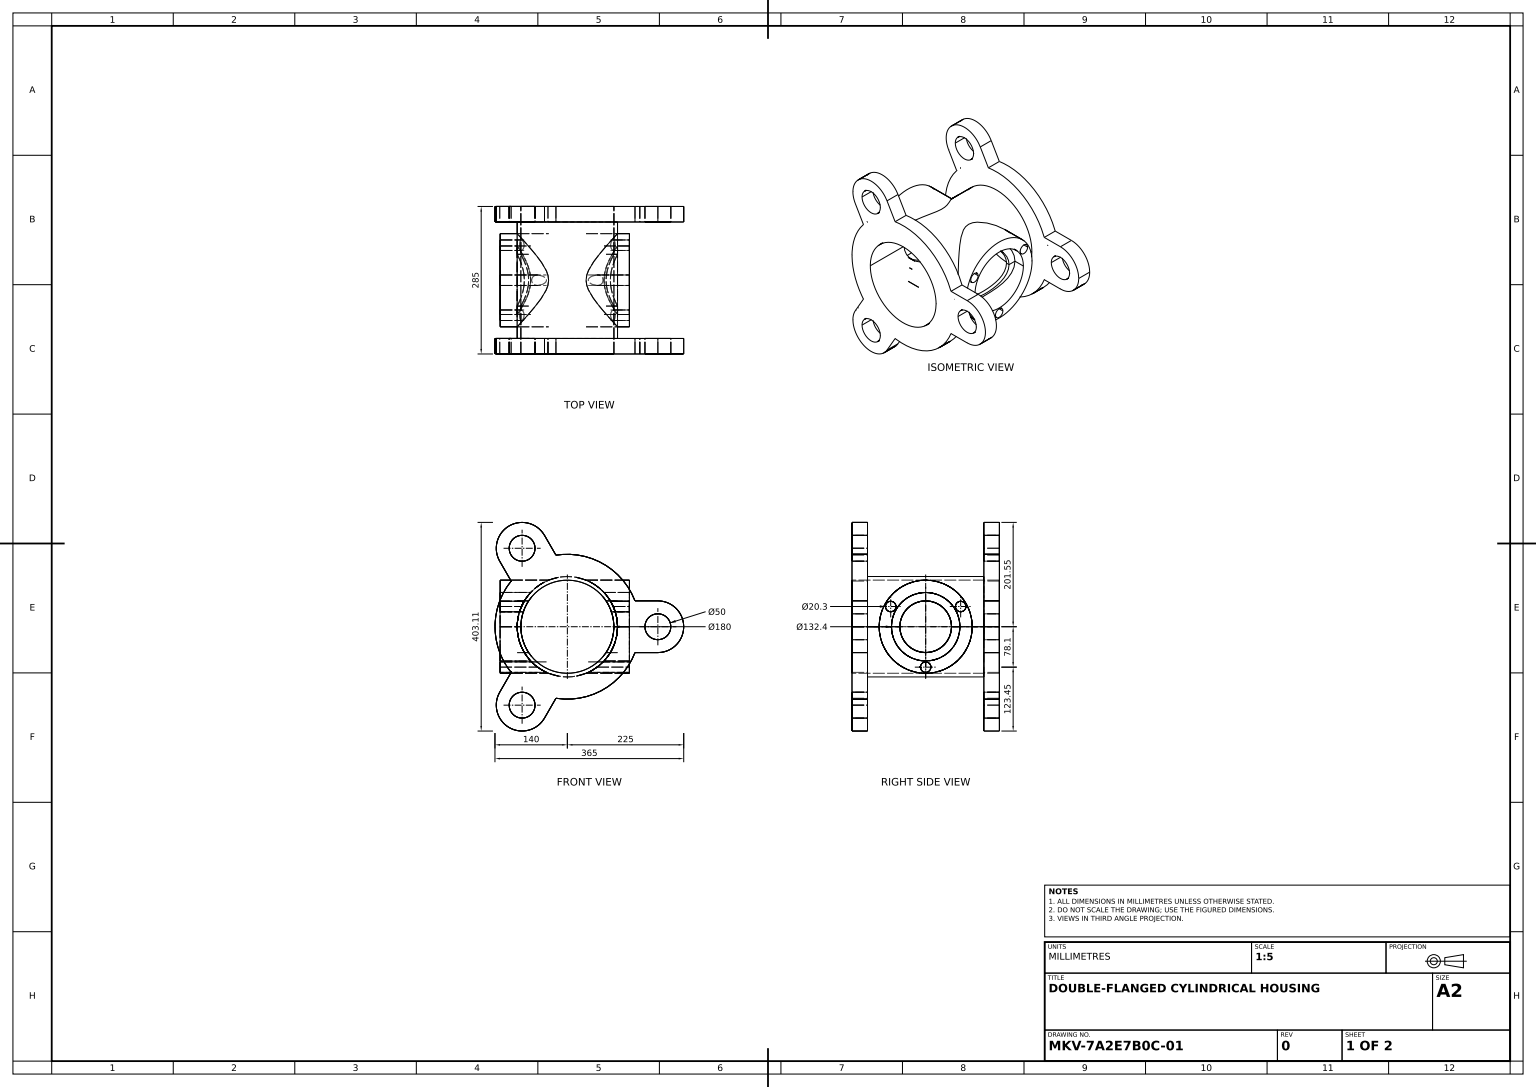
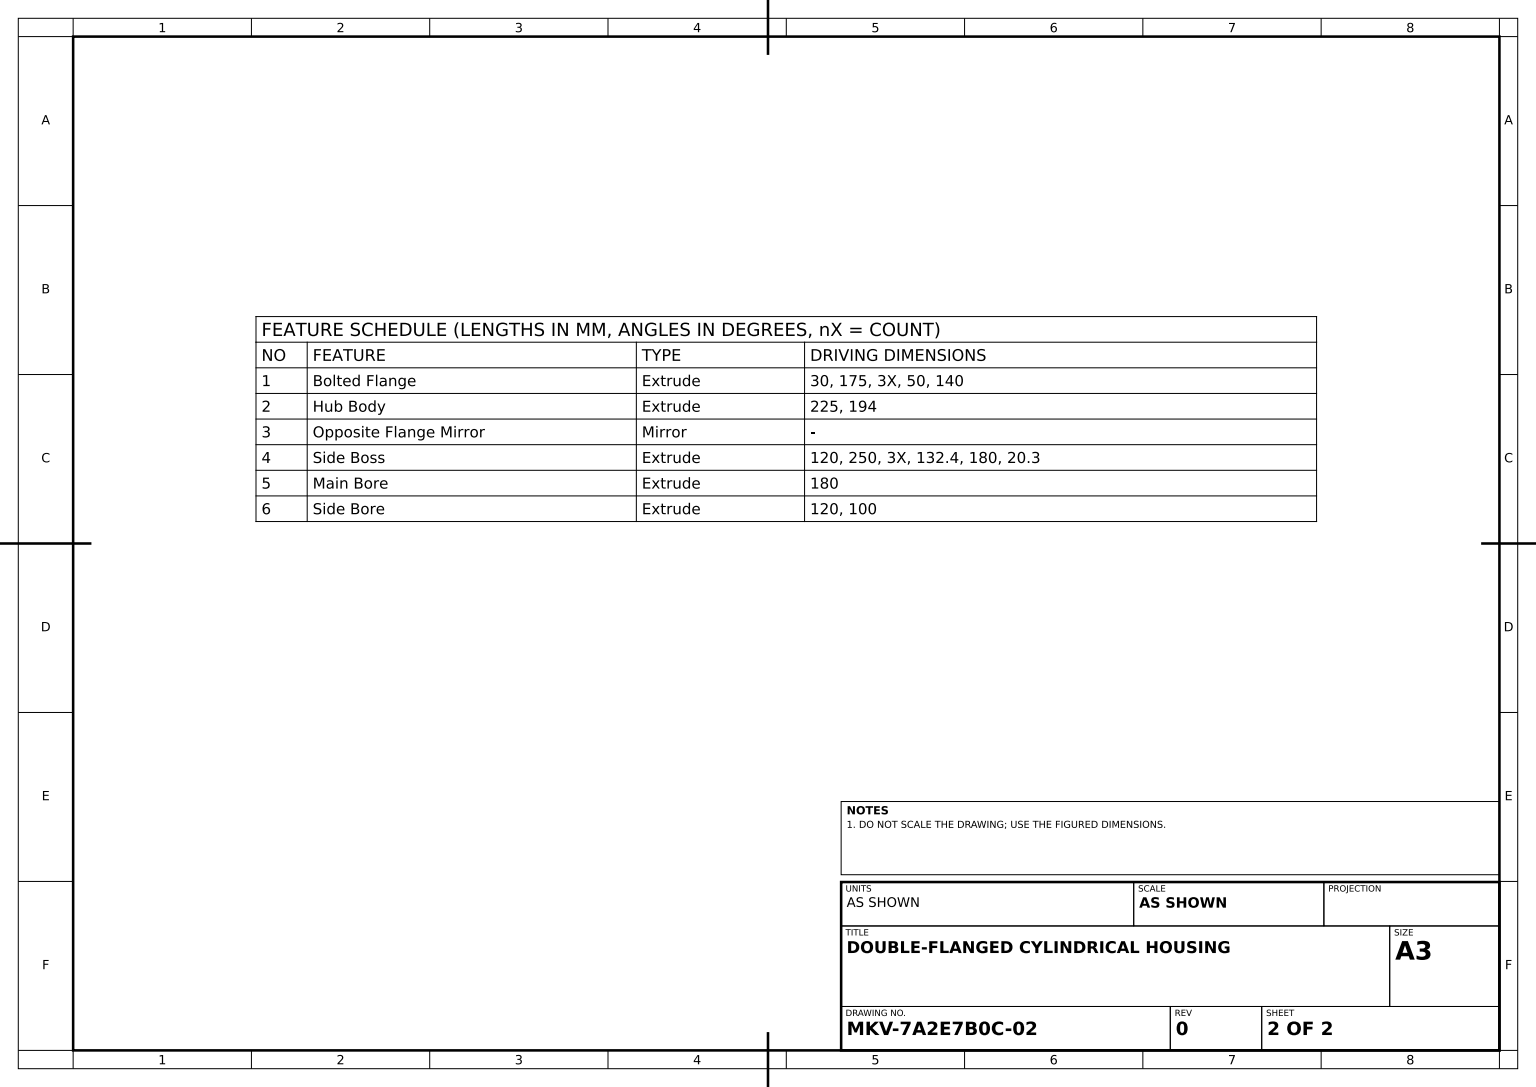
from build123d import *

# Parameters (mm, degrees)
FLANGE_PROFILE_SKETCH_R      = 25
BOLTED_FLANGE_DEPTH          = 30
HUB_PROFILE_SKETCH_R         = 97
HUB_BODY_DEPTH               = 225
SIDE_BOSS_PROFILE_SKETCH_R   = 90
SIDE_BOSS_PROFILE_SKETCH_R_2 = 66.2
SIDE_BOSS_PROFILE_SKETCH_R_3 = 10.15
SIDE_BOSS_DEPTH              = 250
MAIN_BORE_SKETCH_R           = 90
MAIN_BORE_DEPTH              = 416.300125892
SIDE_BORE_SKETCH_R           = 50
SIDE_BORE_DEPTH              = 417.232140237


with BuildPart() as part:
    # Flange Profile Sketch → Bolted Flange (new body)
    with BuildSketch(Plane.XY):
        with BuildLine():
            Line((175, 50), (130.766968306, 50))
            ThreePointArc((130.766968306, 50), (70, 121.24355653), (-22.082213964, 138.247516529))
            Line((-22.082213964, 138.247516529), (-44.198729811, 176.554445662))
            ThreePointArc((-44.198729811, 176.554445662), (-112.5, 194.855715851), (-130.801270189, 126.554445662))
            Line((-130.801270189, 126.554445662), (-108.684754342, 88.247516529))
            ThreePointArc((-108.684754342, 88.247516529), (-140, 0), (-108.684754342, -88.247516529))
            Line((-108.684754342, -88.247516529), (-130.801270189, -126.554445662))
            ThreePointArc((-130.801270189, -126.554445662), (-112.5, -194.855715851), (-44.198729811, -176.554445662))
            Line((-44.198729811, -176.554445662), (-22.082213964, -138.247516529))
            ThreePointArc((-22.082213964, -138.247516529), (70, -121.24355653), (130.766968306, -50))
            Line((130.766968306, -50), (175, -50))
            ThreePointArc((175, -50), (225, 0), (175, 50))
        make_face()
        with Locations((175, 0)):
            Circle(FLANGE_PROFILE_SKETCH_R, mode=Mode.SUBTRACT)
        with Locations((-87.5, -151.554445662)):
            Circle(FLANGE_PROFILE_SKETCH_R, mode=Mode.SUBTRACT)
        with Locations((-87.5, 151.554445662)):
            Circle(FLANGE_PROFILE_SKETCH_R, mode=Mode.SUBTRACT)
    bolted_flange = extrude(amount=BOLTED_FLANGE_DEPTH)

    # Hub Profile Sketch → Hub Body (add)
    with BuildSketch(Plane(origin=(0, 0, 0), x_dir=(-1, 0, 0), z_dir=(0, 0, -1))):
        with Locations(Location((0, 0, 0), (0, 0, 180))):
            Circle(HUB_PROFILE_SKETCH_R)
    extrude(amount=HUB_BODY_DEPTH)

    # Opposite Flange Mirror: Bolted Flange across plane
    add(bolted_flange.mirror(Plane.XY.offset(-112.5)))

    # Side Boss Profile Sketch → Side Boss (add)
    with BuildSketch(Plane(origin=(120, 0, 0), x_dir=(0, 0, -1), z_dir=(1, 0, 0))):
        with Locations((112.5, 0)):
            Circle(SIDE_BOSS_PROFILE_SKETCH_R)
        with Locations((112.5, 0)):
            Circle(SIDE_BOSS_PROFILE_SKETCH_R_2, mode=Mode.SUBTRACT)
        with Locations((112.5, -78.1)):
            Circle(SIDE_BOSS_PROFILE_SKETCH_R_3, mode=Mode.SUBTRACT)
        with Locations((44.863415964, 39.05)):
            Circle(SIDE_BOSS_PROFILE_SKETCH_R_3, mode=Mode.SUBTRACT)
        with Locations((180.136584036, 39.05)):
            Circle(SIDE_BOSS_PROFILE_SKETCH_R_3, mode=Mode.SUBTRACT)
    extrude(amount=-SIDE_BOSS_DEPTH)

    # Main Bore Sketch → Main Bore (cut, through all)
    with BuildSketch(Plane(origin=(0, 0, -255), x_dir=(-1, 0, 0), z_dir=(0, 0, -1))):
        Circle(MAIN_BORE_SKETCH_R)
    extrude(amount=-MAIN_BORE_DEPTH, mode=Mode.SUBTRACT)

    # Side Bore Sketch → Side Bore (cut, through all)
    with BuildSketch(Plane(origin=(120, 0, 0), x_dir=(0, 0, -1), z_dir=(1, 0, 0))):
        with Locations((112.5, 0)):
            Circle(SIDE_BORE_SKETCH_R)
    extrude(amount=-SIDE_BORE_DEPTH, mode=Mode.SUBTRACT)


solid = part.part
